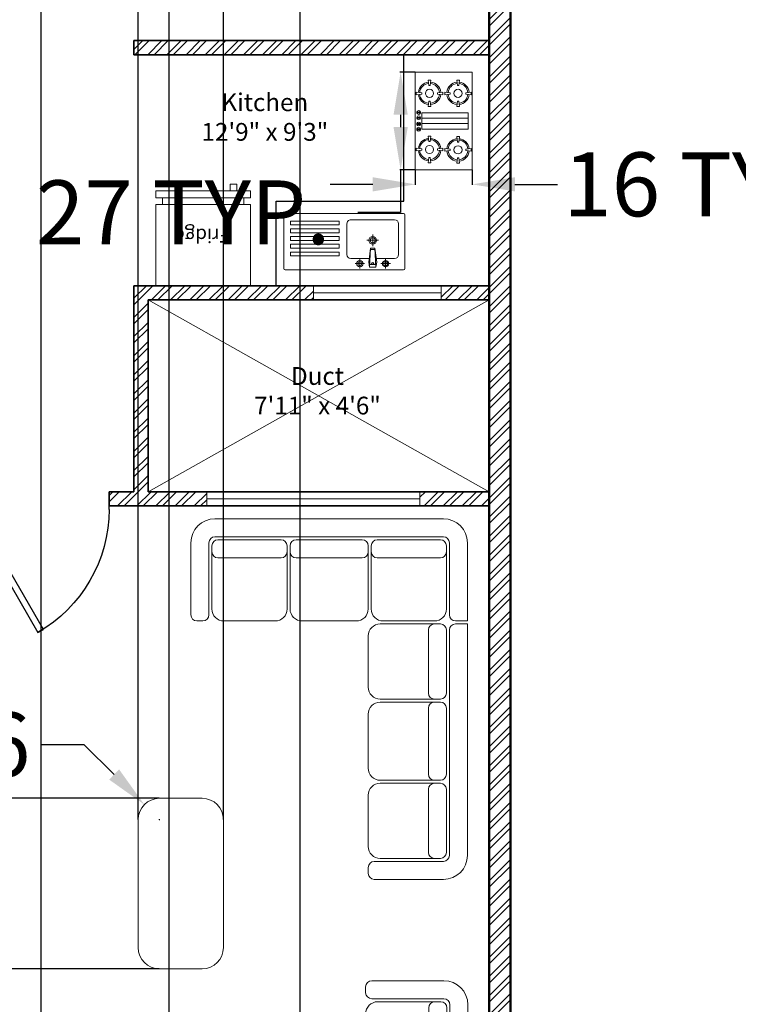
# Model space of a CAD drawing. Units: inches. Extents: x 73 to 1216, y -495 to 328.
# Tile 6 of 9: x 792 to 994, y -232 to 45. Entities that reach past the tile are written whole.
import ezdxf

# ---------------------------------------------------------------- set-up
doc = ezdxf.new("R2010")
doc.units = ezdxf.units.IN
for name, color, linetype, lineweight in [('A-ANNO-DIMS', 2, 'Continuous', 18), ('A-AREA-IDEN', 7, 'Continuous', 18), ('A-DOOR', 3, 'Continuous', 25), ('A-EQPM', 6, 'Continuous', 18), ('A-FLOR-FIXT', 9, 'Continuous', 18), ('A-FLOR-OPEN', 8, 'Continuous', 13), ('A-GLAZ', 3, 'Continuous', 18), ('A-WALL-PATT', 8, 'Continuous', 13), ('Furniture', 2, 'Continuous', 18), ('Inner Walls', 5, 'Continuous', 35), ('Kitchen', 6, 'Continuous', 25), ('Outer Walls', 1, 'Continuous', 50), ('Text-T18', 7, 'Continuous', 18)]:
    doc.layers.add(name, color=color, linetype=linetype, lineweight=lineweight)
doc.styles.get("Standard").update_dxf_attribs({"font": 'arial.ttf'})
doc.dimstyles.get("Standard").update_dxf_attribs({"dimtxt": 18, "dimasz": 12, "dimexe": 0.18, "dimexo": 0.0625, "dimgap": 0.09, "dimtad": 0, "dimtih": 1, "dimtoh": 1, "dimdec": 0, "dimzin": 0, "dimdsep": 46, "dimlunit": 3, "dimtxsty": 'Standard', "dimcen": 0.09, "dimadec": 0, "dimazin": 0, "dimtfac": 1, "dimtdec": 0, "dimtofl": 0, "dimtmove": 0, "dimatfit": 3, "dimfxl": 1, "dimtolj": 1, "dimtzin": 0, "dimarcsym": 0})
pattern_1 = [(45, (-647.324, -1257.0093), (-2.694077, 2.694077), []), (45, (-645.528, -1257.0093), (-2.694077, 2.694077), [])]

# ---------------------------------------------------------------- blocks, each defined once
blk = doc.blocks.new('*U4')
for p, q in [((0, 0), (0, -4)), ((40, 0), (40, -4))]:
    blk.add_line(p, q)
blk.add_lwpolyline([(0, 0), (20, 34.64), (21.52, 33.77), (1.52, -0.88)], close=True)
blk.add_arc((0, 0), 40, 0, 60)
blk = doc.blocks.new('A$C2AFA021D')
for p, q in [((0.8, 2.3), (0.2, 2.3)), ((0.85, 2.2), (0.85, 2.25)), ((0.2, 2.15), (0.8, 2.15)), ((0, 2.1), (0, 0.2)), ((0.15, 0.2), (0.15, 2.1)), ((0.175, 1.55), (0.175, 2.075)), ((0.225, 2.125), (0.275, 2.125)), ((0.75, 2.125), (0.275, 2.125)), ((0.325, 2.075), (0.325, 1.55)), ((0.85, 1.6), (0.85, 2.025)), ((0.275, 1.5), (0.225, 1.5)), ((0.225, 1.475), (0.275, 1.475)), ((0.275, 1.5), (0.75, 1.5)), ((0.75, 1.475), (0.275, 1.475)), ((0.175, 0.875), (0.175, 1.425)), ((0.325, 1.425), (0.325, 0.875)), ((0.85, 0.925), (0.85, 1.375)), ((0.275, 0.825), (0.225, 0.825)), ((0.275, 0.825), (0.75, 0.825)), ((0.975, 0.825), (1.4, 0.825)), ((1.625, 0.825), (2.075, 0.825)), ((2.3, 0.825), (2.725, 0.825)), ((2.9, 0.825), (2.95, 0.825)), ((0.175, 0.225), (0.175, 0.75)), ((0.225, 0.8), (0.275, 0.8)), ((0.75, 0.8), (0.275, 0.8)), ((0.325, 0.75), (0.325, 0.225)), ((2.85, 0.2), (2.85, 0.775)), ((3, 0.775), (3, 0.2)), ((0.85, 0.275), (0.85, 0.7)), ((0.875, 0.275), (0.875, 0.725)), ((1.5, 0.725), (1.5, 0.275)), ((1.525, 0.275), (1.525, 0.725)), ((2.175, 0.725), (2.175, 0.275)), ((2.2, 0.275), (2.2, 0.725)), ((2.825, 0.725), (2.825, 0.275)), ((0.875, 0.275), (0.875, 0.225)), ((1.45, 0.325), (0.925, 0.325)), ((1.5, 0.225), (1.5, 0.275)), ((1.525, 0.275), (1.525, 0.225)), ((2.125, 0.325), (1.575, 0.325)), ((2.175, 0.225), (2.175, 0.275)), ((2.2, 0.275), (2.2, 0.225)), ((2.775, 0.325), (2.25, 0.325)), ((2.825, 0.225), (2.825, 0.275)), ((0.275, 0.175), (0.225, 0.175)), ((0.275, 0.175), (0.75, 0.175)), ((0.925, 0.175), (1.45, 0.175)), ((1.575, 0.175), (2.125, 0.175)), ((2.25, 0.175), (2.775, 0.175)), ((0.8, 0.15), (0.2, 0.15)), ((0.85, 0), (0.85, 0.1)), ((0.875, 0.1), (0.875, 0)), ((0.925, 0.15), (2.8, 0.15)), ((0.2, 0), (0.85, 0)), ((2.8, 0), (0.875, 0))]:
    blk.add_line(p, q)
for centre, radius, start, end in [((0.2, 2.1), 0.2, 90, 180), ((0.8, 2.25), 0.05, 0, 90), ((0.2, 2.1), 0.05, 90, 180), ((0.8, 2.2), 0.05, 270, 0), ((0.225, 2.075), 0.05, 90, 180), ((0.275, 2.075), 0.05, 0, 90), ((0.75, 2.025), 0.1, 0, 90), ((0.75, 1.6), 0.1, 270, 0), ((0.225, 1.55), 0.05, 180, 270), ((0.225, 1.425), 0.05, 90, 180), ((0.275, 1.55), 0.05, 270, 0), ((0.275, 1.425), 0.05, 0, 90), ((0.75, 1.375), 0.1, 360, 90), ((0.75, 0.925), 0.1, 270, 0), ((0.225, 0.875), 0.05, 180, 270), ((0.275, 0.875), 0.05, 270, 0), ((0.975, 0.725), 0.1, 90, 180), ((1.4, 0.725), 0.1, 0, 90), ((1.625, 0.725), 0.1, 90, 180), ((2.075, 0.725), 0.1, 0, 90), ((2.3, 0.725), 0.1, 90, 180), ((2.725, 0.725), 0.1, 0, 90), ((2.9, 0.775), 0.05, 90, 180), ((2.95, 0.775), 0.05, 0, 90), ((0.225, 0.75), 0.05, 90, 180), ((0.275, 0.75), 0.05, 0, 90), ((0.75, 0.7), 0.1, 0, 90), ((0.75, 0.275), 0.1, 270, 0), ((0.925, 0.275), 0.05, 90, 180), ((1.45, 0.275), 0.05, 360, 90), ((1.575, 0.275), 0.05, 90, 180), ((2.125, 0.275), 0.05, 360, 90), ((2.25, 0.275), 0.05, 90, 180), ((2.775, 0.275), 0.05, 360, 90), ((0.2, 0.2), 0.2, 180, 270), ((0.2, 0.2), 0.05, 180, 270), ((0.225, 0.225), 0.05, 180, 270), ((0.275, 0.225), 0.05, 270, 0), ((0.925, 0.225), 0.05, 180, 270), ((1.45, 0.225), 0.05, 270, 0), ((1.575, 0.225), 0.05, 180, 270), ((2.125, 0.225), 0.05, 270, 0), ((2.25, 0.225), 0.05, 180, 270), ((2.775, 0.225), 0.05, 270, 0), ((2.8, 0.2), 0.2, 270, 0), ((2.8, 0.2), 0.05, 270, 0), ((0.8, 0.1), 0.05, 0, 90), ((0.925, 0.1), 0.05, 90, 180)]:
    blk.add_arc(centre, radius, start, end)
blk = doc.blocks.new('A$C57CF26DA')
for p, q in [((0, 0), (0, 420)), ((720, 420), (0, 420)), ((166.9, 413), (146.9, 413)), ((146.9, 413), (151.9, 373)), ((151.9, 373), (161.9, 373)), ((161.9, 373), (166.9, 413)), ((300, 390.9), (300, 49.1)), ((300, 390.9), (420, 390.9)), ((340, 390.9), (340, 49.1)), ((380, 390.9), (380, 49.1)), ((420, 390.9), (420, 49.1)), ((583.6, 413), (563.6, 413)), ((563.6, 413), (568.6, 373)), ((568.6, 373), (578.6, 373)), ((578.6, 373), (583.6, 413)), ((720, 0), (720, 420)), ((98.9, 320), (58.9, 325)), ((58.9, 325), (58.9, 305)), ((58.9, 305), (98.9, 310)), ((98.9, 310), (98.9, 320)), ((254.8, 325), (214.8, 320)), ((214.8, 320), (214.8, 310)), ((214.8, 310), (254.8, 305)), ((254.8, 305), (254.8, 325)), ((515.6, 320), (475.6, 325)), ((475.6, 325), (475.6, 305)), ((475.6, 305), (515.6, 310)), ((515.6, 310), (515.6, 320)), ((671.6, 325), (631.6, 320)), ((631.6, 320), (631.6, 310)), ((631.6, 310), (671.6, 305)), ((671.6, 305), (671.6, 325)), ((151.9, 257), (146.9, 217)), ((161.9, 257), (151.9, 257)), ((166.9, 217), (161.9, 257)), ((568.6, 257), (563.6, 217)), ((578.6, 257), (568.6, 257)), ((583.6, 217), (578.6, 257)), ((146.9, 217), (166.9, 217)), ((166.9, 203), (146.9, 203)), ((146.9, 203), (151.9, 163)), ((151.9, 163), (161.9, 163)), ((161.9, 163), (166.9, 203)), ((581.1, 203), (561.1, 203)), ((561.1, 203), (566.1, 163)), ((563.6, 217), (583.6, 217)), ((566.1, 163), (576.1, 163)), ((576.1, 163), (581.1, 203)), ((98.9, 110), (58.9, 115)), ((58.9, 115), (58.9, 95)), ((58.9, 95), (98.9, 100)), ((98.9, 100), (98.9, 110)), ((254.8, 115), (214.8, 110)), ((214.8, 110), (214.8, 100)), ((214.8, 100), (254.8, 95)), ((254.8, 95), (254.8, 115)), ((513.1, 110), (473.1, 115)), ((473.1, 115), (473.1, 95)), ((473.1, 95), (513.1, 100)), ((513.1, 100), (513.1, 110)), ((669, 115), (629, 110)), ((629, 110), (629, 100)), ((629, 100), (669, 95)), ((669, 95), (669, 115)), ((151.9, 47), (146.9, 7)), ((146.9, 7), (166.9, 7)), ((161.9, 47), (151.9, 47)), ((166.9, 7), (161.9, 47)), ((301.5, 38.7), (294.7, 38.7)), ((294.7, 38.7), (294.7, 11.3)), ((294.7, 11.3), (301.5, 11.3)), ((420, 49.1), (300, 49.1)), ((301.5, 11.3), (301.5, 38.7)), ((340.5, 38.7), (333.7, 38.7)), ((333.7, 38.7), (333.7, 11.3)), ((333.7, 11.3), (340.5, 11.3)), ((340.5, 11.3), (340.5, 38.7)), ((379.7, 11.3), (379.7, 38.7)), ((379.7, 38.7), (386.5, 38.7)), ((386.5, 11.3), (379.7, 11.3)), ((386.5, 38.7), (386.5, 11.3)), ((418.7, 11.3), (418.7, 38.7)), ((418.7, 38.7), (425.5, 38.7)), ((425.5, 11.3), (418.7, 11.3)), ((425.5, 38.7), (425.5, 11.3)), ((566.1, 47), (561.1, 7)), ((561.1, 7), (581.1, 7)), ((576.1, 47), (566.1, 47)), ((581.1, 7), (576.1, 47)), ((720, 0), (0, 0))]:
    blk.add_line(p, q)
for centre in [(156.9, 315), (573.6, 315), (156.9, 105), (571.1, 105)]:
    blk.add_circle(centre, 30)
for centre, radius, start, end in [((156.9, 315), 83, 95.58493, 174.41507), ((156.9, 315), 73, 95.37384, 174.62616), ((156.9, 315), 73, 5.37384, 84.62616), ((156.9, 315), 83, 5.58493, 84.41507), ((573.6, 315), 83, 95.58493, 174.41507), ((573.6, 315), 73, 95.37384, 174.62616), ((573.6, 315), 73, 5.37384, 84.62616), ((573.6, 315), 83, 5.58493, 84.41507), ((156.9, 315), 83, 185.58493, 264.41507), ((156.9, 315), 73, 185.37384, 264.62616), ((156.9, 315), 73, 275.37384, 354.62616), ((156.9, 315), 83, 275.58493, 354.41507), ((573.6, 315), 83, 185.58493, 264.41507), ((573.6, 315), 73, 185.37384, 264.62616), ((573.6, 315), 73, 275.37384, 354.62616), ((573.6, 315), 83, 275.58493, 354.41507), ((156.9, 105), 83, 95.58493, 174.41507), ((156.9, 105), 73, 95.37384, 174.62616), ((156.9, 105), 73, 5.37384, 84.62616), ((156.9, 105), 83, 5.58493, 84.41507), ((571.1, 105), 83, 95.58493, 174.41507), ((571.1, 105), 73, 95.37384, 174.62616), ((571.1, 105), 73, 5.37384, 84.62616), ((571.1, 105), 83, 5.58493, 84.41507), ((156.9, 105), 83, 185.58493, 264.41507), ((156.9, 105), 73, 185.37384, 264.62616), ((156.9, 105), 73, 275.37384, 354.62616), ((156.9, 105), 83, 275.58493, 354.41507), ((571.1, 105), 83, 185.58493, 264.41507), ((571.1, 105), 73, 185.37384, 264.62616), ((571.1, 105), 73, 275.37384, 354.62616), ((571.1, 105), 83, 275.58493, 354.41507), ((298.1, 25), 13.7, 104.47751, 255.52249), ((298.1, 25), 13.7, 284.47751, 75.52249), ((337.1, 25), 13.7, 104.47751, 255.52249), ((337.1, 25), 13.7, 284.47751, 75.52249), ((383.1, 25), 13.7, 104.47751, 255.52249), ((383.1, 25), 13.7, 284.47751, 75.52249), ((422.1, 25), 13.7, 104.47751, 255.52249), ((422.1, 25), 13.7, 284.47751, 75.52249)]:
    blk.add_arc(centre, radius, start, end)
blk = doc.blocks.new('A$C7C492201')
for p, q in [((0, 10), (0, 426.6)), ((10, 436.6), (927.3, 436.6)), ((111.9, 388.7), (185, 388.7)), ((148.5, 425.2), (148.5, 352.2)), ((223.5, 415), (217, 376.2)), ((223.5, 415), (231.8, 268.5)), ((223.5, 415), (248.5, 415)), ((224.6, 395.4), (248.5, 395.4)), ((273.5, 415), (248.5, 415)), ((272.3, 395.4), (248.5, 395.4)), ((273.5, 415), (265.2, 268.5)), ((273.5, 415), (279.9, 376.2)), ((311.9, 388.7), (385, 388.7)), ((348.5, 425.2), (348.5, 352.2)), ((937.3, 10), (937.3, 426.6)), ((48.5, 318.8), (48.5, 78.8)), ((220.8, 348.8), (78.5, 348.8)), ((217, 376.2), (231.8, 268.5)), ((279.9, 376.2), (265.2, 268.5)), ((418.5, 348.8), (276.2, 348.8)), ((448.5, 318.8), (448.5, 78.8)), ((509.1, 328.4), (509.1, 298.4)), ((509.1, 328.4), (885, 328.4)), ((885, 328.4), (885, 298.4)), ((231.3, 278.6), (248.5, 278.6)), ((231.8, 268.5), (248.5, 268.5)), ((265.6, 278.6), (248.5, 278.6)), ((265.2, 268.5), (248.5, 268.5)), ((248.5, 252.8), (248.5, 162.6)), ((509.1, 298.4), (885, 298.4)), ((509.1, 268.4), (509.1, 238.4)), ((509.1, 268.4), (885, 268.4)), ((509.1, 238.4), (885, 238.4)), ((885, 268.4), (885, 238.4)), ((203.4, 207.7), (293.5, 207.7)), ((509.1, 208.4), (885, 208.4)), ((509.1, 208.4), (509.1, 178.4)), ((509.1, 178.4), (885, 178.4)), ((885, 208.4), (885, 178.4)), ((509.1, 148.4), (509.1, 118.4)), ((509.1, 148.4), (885, 148.4)), ((509.1, 118.4), (885, 118.4)), ((509.1, 88.4), (509.1, 58.4)), ((509.1, 88.4), (885, 88.4)), ((885, 148.4), (885, 118.4)), ((885, 88.4), (885, 58.4)), ((927.3, 0), (10, 0)), ((418.5, 48.8), (78.5, 48.8)), ((509.1, 58.4), (885, 58.4))]:
    blk.add_line(p, q)
for centre, radius in [((148.5, 388.7), 25), ((148.5, 388.7), 15), ((348.5, 388.7), 25), ((348.5, 388.7), 15), ((248.5, 207.7), 30), ((248.5, 207.7), 20)]:
    blk.add_circle(centre, radius)
for centre, radius, start, end in [((10, 426.6), 10, 90, 180), ((247.3, 388), 7.19, 80.52523, 279.47477), ((249.6, 388), 7.19, 260.52523, 99.47477), ((927.3, 426.6), 10, 0, 90), ((78.5, 318.8), 30, 90, 180), ((418.5, 318.8), 30, 0, 90), ((78.5, 78.8), 30, 180, 270), ((418.5, 78.8), 30, 270, 0), ((10, 10), 10, 180, 270), ((927.3, 10), 10, 270, 0)]:
    blk.add_arc(centre, radius, start, end)
blk = doc.blocks.new('REFRI-00')
for points in [[(-0.35, 0.35), (-0.35, -0.25), (0.35, -0.25), (0.35, 0.35), (-0.35, 0.35)], [(-0.3, -0.3), (-0.3, -0.25)], [(0.3, -0.3), (0.3, -0.25)], [(-0.35, -0.3), (-0.35, -0.35), (0.35, -0.35), (0.35, -0.3), (-0.35, -0.3)], [(-0.25, -0.35), (-0.25, -0.4), (-0.2, -0.4), (-0.2, -0.35)]]:
    blk.add_lwpolyline(points)
blk = doc.blocks.new('*D26')
at = {"layer": 'A-ANNO-DIMS', "color": 0, "lineweight": -2, "transparency": 16777216}
for p, q in [((690.69, 91.4), (690.69, 79.21)), ((771.16, 91.4), (771.16, 79.21)), ((702.69, 79.39), (759.16, 79.39)), ((771.16, 79.39), (783.16, 79.39))]:
    blk.add_line(p, q, dxfattribs=at)
at = {"layer": 'A-ANNO-DIMS', "color": 0, "transparency": 16777216}
for points in [[(702.69, 81.39), (702.69, 77.39), (690.69, 79.39)], [(759.16, 81.39), (759.16, 77.39), (771.16, 79.39)]]:
    blk.add_solid(points, dxfattribs=at)
at = {"layer": 'Defpoints', "color": 0, "transparency": 16777216}
for p in [(690.69, 91.46), (771.16, 91.46), (771.16, 79.39)]:
    blk.add_point(p, dxfattribs=at)
at = {"layer": 'A-ANNO-DIMS', "color": 0, "transparency": 16777216, "insert": (890.24, 79.39), "char_height": 18, "attachment_point": 5}
blk.add_mtext('\\A1;KING BED 80 TYP.', dxfattribs=at)
blk = doc.blocks.new('*D38')
at = {"layer": 'A-ANNO-DIMS', "color": 0, "lineweight": -2, "transparency": 16777216}
for p, q in [((835.16, 83.11), (835.16, 69.65)), ((924.16, 83.11), (924.16, 69.65)), ((847.16, 69.83), (912.16, 69.83)), ((924.16, 69.83), (936.16, 69.83))]:
    blk.add_line(p, q, dxfattribs=at)
at = {"layer": 'A-ANNO-DIMS', "color": 0, "transparency": 16777216}
for points in [[(847.16, 71.83), (847.16, 67.83), (835.16, 69.83)], [(912.16, 71.83), (912.16, 67.83), (924.16, 69.83)]]:
    blk.add_solid(points, dxfattribs=at)
at = {"layer": 'Defpoints', "color": 0, "transparency": 16777216}
for p in [(835.16, 83.18), (924.16, 83.18), (924.16, 69.83)]:
    blk.add_point(p, dxfattribs=at)
at = {"layer": 'A-ANNO-DIMS', "color": 0, "transparency": 16777216, "insert": (1057.97, 69.83), "char_height": 18, "attachment_point": 5}
blk.add_mtext('\\A1;WARDROBE 89 TYP.', dxfattribs=at)
blk = doc.blocks.new('*D42')
at = {"layer": 'A-ANNO-DIMS', "color": 0, "lineweight": -2, "transparency": 16777216}
for p, q in [((903.29, 30.3), (899.05, 30.3)), ((899.23, 18.3), (899.23, 14.82)), ((903.29, 2.82), (899.05, 2.82)), ((899.23, 2.82), (899.23, -9.18)), ((899.23, -9.18), (887.23, -9.18))]:
    blk.add_line(p, q, dxfattribs=at)
at = {"layer": 'A-ANNO-DIMS', "color": 0, "transparency": 16777216}
for points in [[(897.23, 18.3), (901.23, 18.3), (899.23, 30.3)], [(897.23, 14.82), (901.23, 14.82), (899.23, 2.82)]]:
    blk.add_solid(points, dxfattribs=at)
at = {"layer": 'Defpoints', "color": 0, "transparency": 16777216}
for p in [(903.36, 30.3), (899.23, 2.82), (903.36, 2.82)]:
    blk.add_point(p, dxfattribs=at)
at = {"layer": 'A-ANNO-DIMS', "color": 0, "transparency": 16777216, "insert": (777.07, -9.18), "char_height": 18, "attachment_point": 5}
blk.add_mtext('\\A1;COOKTOP 27 TYP.', dxfattribs=at)
blk = doc.blocks.new('*D43')
at = {"layer": 'A-ANNO-DIMS', "color": 0, "lineweight": -2, "transparency": 16777216}
for p, q in [((903.36, 2.76), (903.36, -1.48)), ((919.39, 2.76), (919.39, -1.48)), ((891.36, -1.3), (879.36, -1.3)), ((931.39, -1.3), (943.39, -1.3))]:
    blk.add_line(p, q, dxfattribs=at)
at = {"layer": 'A-ANNO-DIMS', "color": 0, "transparency": 16777216}
for points in [[(891.36, 0.7), (891.36, -3.3), (903.36, -1.3)], [(931.39, 0.7), (931.39, -3.3), (919.39, -1.3)]]:
    blk.add_solid(points, dxfattribs=at)
at = {"layer": 'Defpoints', "color": 0, "transparency": 16777216}
for p in [(903.36, 2.82), (919.39, 2.82), (919.39, -1.3)]:
    blk.add_point(p, dxfattribs=at)
at = {"layer": 'A-ANNO-DIMS', "color": 0, "transparency": 16777216, "insert": (986.44, -1.3), "char_height": 18, "attachment_point": 5}
blk.add_mtext('\\A1;16 TYP.', dxfattribs=at)
blk = doc.blocks.new('*D67')
at = {"layer": 'A-ANNO-DIMS', "color": 0, "lineweight": -2, "transparency": 16777216}
for p, q in [((798.02113, 227.113801), (798.02113, -465.403699)), ((834.02113, 227.113801), (834.02113, -465.403699)), ((786.02113, -465.223699), (774.02113, -465.223699)), ((846.02113, -465.223699), (858.02113, -465.223699))]:
    blk.add_line(p, q, dxfattribs=at)
at = {"layer": 'A-ANNO-DIMS', "color": 0, "transparency": 16777216}
for points in [[(786.02113, -463.223699), (786.02113, -467.223699), (798.02113, -465.223699)], [(846.02113, -463.223699), (846.02113, -467.223699), (834.02113, -465.223699)]]:
    blk.add_solid(points, dxfattribs=at)
at = {"layer": 'Defpoints', "color": 0, "transparency": 16777216}
for p in [(798.02113, 227.176301), (834.02113, 227.176301), (834.02113, -465.223699)]:
    blk.add_point(p, dxfattribs=at)
at = {"layer": 'A-ANNO-DIMS', "color": 0, "transparency": 16777216, "insert": (816.02113, -465.223699), "char_height": 18, "attachment_point": 5}
blk.add_mtext('\\A1;36', dxfattribs=at)
blk = doc.blocks.new('*D68')
at = {"layer": 'A-ANNO-DIMS', "color": 0, "lineweight": -2, "transparency": 16777216}
for p, q in [((834.02, 227.11), (834.02, -465.4)), ((870.82, 227.11), (870.82, -465.4)), ((846.02, -465.22), (858.82, -465.22)), ((870.82, -465.22), (882.82, -465.22))]:
    blk.add_line(p, q, dxfattribs=at)
at = {"layer": 'A-ANNO-DIMS', "color": 0, "transparency": 16777216}
for points in [[(846.02, -463.22), (846.02, -467.22), (834.02, -465.22)], [(858.82, -463.22), (858.82, -467.22), (870.82, -465.22)]]:
    blk.add_solid(points, dxfattribs=at)
at = {"layer": 'Defpoints', "color": 0, "transparency": 16777216}
for p in [(834.02, 227.18), (870.82, 227.18), (870.82, -465.22)]:
    blk.add_point(p, dxfattribs=at)
at = {"layer": 'A-ANNO-DIMS', "color": 0, "transparency": 16777216, "insert": (906.3, -465.22), "char_height": 18, "attachment_point": 5}
blk.add_mtext('\\A1;36.8', dxfattribs=at)
blk = doc.blocks.new('*D77')
at = {"layer": 'A-ANNO-DIMS', "color": 0, "lineweight": -2, "transparency": 16777216}
for p, q in [((813.36, 316.58), (801.36, 316.58)), ((825.36, -180.08), (825.36, 316.76)), ((849.36, -180.08), (849.36, 316.76)), ((861.36, 316.58), (873.36, 316.58))]:
    blk.add_line(p, q, dxfattribs=at)
at = {"layer": 'A-ANNO-DIMS', "color": 0, "transparency": 16777216}
for points in [[(813.36, 318.58), (813.36, 314.58), (825.36, 316.58)], [(861.36, 318.58), (861.36, 314.58), (849.36, 316.58)]]:
    blk.add_solid(points, dxfattribs=at)
at = {"layer": 'Defpoints', "color": 0, "transparency": 16777216}
for p in [(849.36, 316.58), (825.36, -180.14), (849.36, -180.14)]:
    blk.add_point(p, dxfattribs=at)
at = {"layer": 'A-ANNO-DIMS', "color": 0, "transparency": 16777216, "insert": (886.46, 316.58), "char_height": 18, "attachment_point": 5}
blk.add_mtext('\\A1;24', dxfattribs=at)
blk = doc.blocks.new('*D78')
at = {"layer": 'A-ANNO-DIMS', "color": 0, "lineweight": -2, "transparency": 16777216}
for p, q in [((831.3, -174.14), (542.58, -174.14)), ((542.76, -186.14), (542.76, -188.86)), ((542.76, -210.14), (542.76, -207.42)), ((831.3, -222.14), (542.58, -222.14))]:
    blk.add_line(p, q, dxfattribs=at)
at = {"layer": 'A-ANNO-DIMS', "color": 0, "transparency": 16777216}
for points in [[(540.76, -186.14), (544.76, -186.14), (542.76, -174.14)], [(540.76, -210.14), (544.76, -210.14), (542.76, -222.14)]]:
    blk.add_solid(points, dxfattribs=at)
at = {"layer": 'Defpoints', "color": 0, "transparency": 16777216}
for p in [(542.76, -174.14), (831.36, -174.14), (831.36, -222.14)]:
    blk.add_point(p, dxfattribs=at)
at = {"layer": 'A-ANNO-DIMS', "color": 0, "transparency": 16777216, "insert": (542.76, -198.14), "char_height": 18, "attachment_point": 5}
blk.add_mtext('\\A1;48', dxfattribs=at)
blk = doc.blocks.new('*D79')
at = {"layer": 'A-ANNO-DIMS', "color": 0, "lineweight": -2, "transparency": 16777216}
for p, q in [((798.1, -158.97), (810.1, -158.97)), ((810.1, -158.97), (818.61, -167.44)), ((831.27, -180.14), (831.45, -180.14)), ((831.36, -180.23), (831.36, -180.05))]:
    blk.add_line(p, q, dxfattribs=at)
at = {"layer": 'A-ANNO-DIMS', "color": 0, "transparency": 16777216}
blk.add_solid([(820.02, -166.02), (817.19, -168.86), (827.11, -175.91)], dxfattribs=at)
at = {"layer": 'Defpoints', "color": 0, "transparency": 16777216}
for p in [(827.11, -175.91), (831.36, -180.14)]:
    blk.add_point(p, dxfattribs=at)
at = {"layer": 'A-ANNO-DIMS', "color": 0, "transparency": 16777216, "insert": (763.81, -158.97), "char_height": 18, "attachment_point": 5}
blk.add_mtext('\\A1;4X R6', dxfattribs=at)

msp = doc.modelspace()

# ---------------------------------------------------------------- hatches: boundary and pattern name
at = {"layer": 'A-WALL-PATT'}
h = msp.add_hatch(dxfattribs=at)
h.set_pattern_fill('ANSI32', color=256, scale=0.4)
h.set_pattern_definition(pattern_1)
h.paths.add_polyline_path([(586.1647, 273.1763), (924.1647, 273.1763), (924.1647, -421.8237), (753.1647, -421.8237), (753.1647, -427.8237), (930.1647, -427.8237), (930.1647, 279.1763), (580.1647, 279.1763), (580.1647, -427.8237), (633.1647, -427.8237), (633.1647, -421.8237), (586.1647, -421.8237)])
h = msp.add_hatch(dxfattribs=at)
h.set_pattern_fill('ANSI32', color=256, scale=0.4)
h.set_pattern_definition(pattern_1)
h.paths.add_polyline_path([(685.1647, 201.1763), (679.1647, 201.1763), (679.1647, 206.1763), (675.1647, 206.1763), (675.1647, 201.1763), (586.1647, 201.1763), (586.1647, 197.1763), (685.1647, 197.1763)])
h.paths.add_polyline_path([(679.1647, 273.1763), (675.1647, 273.1763), (675.1647, 236.1763), (679.1647, 236.1763)])
h.paths.add_polyline_path([(775.1647, 201.1763), (772.1647, 201.1763), (772.1647, 273.1763), (768.1647, 273.1763), (768.1647, 249.1763), (768.1647, 201.1763), (721.1647, 201.1763), (721.1647, 197.1763), (771.1647, 197.1763), (771.1647, 58.1763), (775.1647, 58.1763)])
h.paths.add_polyline_path([(798.0211, 233.1763), (772.1647, 233.1763), (772.1647, 227.1763), (798.0211, 227.1763)])
h.paths.add_polyline_path([(870.8232, 233.1763), (834.0211, 233.1763), (834.0211, 227.1763), (870.8232, 227.1763)])
h.paths.add_polyline_path([(924.1647, 233.1763), (906.8232, 233.1763), (906.8232, 227.1763), (924.1647, 227.1763)])
h.paths.add_polyline_path([(924.1647, 83.1763), (775.1647, 83.1763), (775.1647, 79.1763), (924.1647, 79.1763)])
h.paths.add_polyline_path([(775.1647, 22.1763), (771.1647, 22.1763), (771.1647, 16.1763), (628.1647, 16.1763), (628.1647, 12.1763), (775.1647, 12.1763)])
h.paths.add_polyline_path([(692.1647, 12.1763), (688.1647, 12.1763), (688.1647, -52.8237), (692.1647, -52.8237)])
h.paths.add_polyline_path([(924.1647, 39.1763), (824.1647, 39.1763), (824.1647, 35.1763), (924.1647, 35.1763)])
h.paths.add_polyline_path([(874.6647, -29.8237), (864.1647, -29.8237), (824.1647, -29.8237), (824.1647, -87.8237), (817.1647, -87.8237), (817.1647, -91.8237), (844.6647, -91.8237), (844.6647, -87.8237), (828.1647, -87.8237), (828.1647, -33.8237), (874.6647, -33.8237)])
h.paths.add_polyline_path([(924.1647, -29.8237), (910.6647, -29.8237), (910.6647, -33.8237), (924.1647, -33.8237)])
h.paths.add_polyline_path([(924.1647, -87.8237), (904.6647, -87.8237), (904.6647, -91.8237), (924.1647, -91.8237)])
h.paths.add_polyline_path([(777.1647, -88.8237), (761.1647, -88.8237), (761.1647, -92.8237), (767.1647, -92.8237), (767.1647, -224.8237), (771.1647, -224.8237), (771.1647, -92.8237), (777.1647, -92.8237)])
h.paths.add_polyline_path([(725.1647, -88.8237), (628.1647, -88.8237), (628.1647, -92.8237), (725.1647, -92.8237)])
h.paths.add_polyline_path([(692.1647, -82.8237), (688.1647, -82.8237), (688.1647, -88.8237), (692.1647, -88.8237)])
h.paths.add_polyline_path([(767.1647, -313.8237), (924.1647, -313.8237), (924.1647, -307.8237), (763.1647, -307.8237), (763.1647, -421.8237), (767.1647, -421.8237)])

# ---------------------------------------------------------------- linework, layer by layer
at = {"layer": 'A-FLOR-OPEN'}
for p, q in [((828.1647, -87.8237), (924.1647, -33.8237)), ((828.1647, -33.8237), (924.1647, -87.8237))]:
    msp.add_line(p, q, dxfattribs=at)
at = {"layer": 'A-GLAZ'}
for p, q in [((874.6647, -33.8237), (874.6647, -29.8237)), ((910.6647, -33.8237), (910.6647, -29.8237)), ((910.6647, -31.8237), (874.6647, -31.8237)), ((844.6647, -91.8237), (844.6647, -87.8237)), ((904.6647, -91.8237), (904.6647, -87.8237)), ((904.6647, -89.8237), (844.6647, -89.8237))]:
    msp.add_line(p, q, dxfattribs=at)
at = {"layer": 'Furniture'}
msp.add_lwpolyline([(831.3578, -174.1414), (843.3578, -174.1414, -0.41421356), (849.3578, -180.1414), (849.3578, -216.1414, -0.41421356), (843.3578, -222.1414), (831.3578, -222.1414, -0.41421356), (825.3578, -216.1414), (825.3578, -180.1414, -0.41421356)], format="xyb", close=True, dxfattribs=at)
at = {"layer": 'Inner Walls'}
for p, q in [((824.1647, 39.1763), (924.1647, 39.1763)), ((824.1647, 39.1763), (824.1647, 35.1763)), ((824.1647, 35.1763), (924.1647, 35.1763)), ((924.1647, -29.8237), (824.1647, -29.8237)), ((824.1647, -87.8237), (824.1647, -29.8237)), ((924.1647, -33.8237), (828.1647, -33.8237)), ((828.1647, -87.8237), (828.1647, -33.8237)), ((824.1647, -87.8237), (817.1647, -87.8237)), ((817.1647, -87.8237), (817.1647, -91.8237)), ((924.1647, -87.8237), (828.1647, -87.8237)), ((924.1647, -91.8237), (817.1647, -91.8237))]:
    msp.add_line(p, q, dxfattribs=at)
at = {"layer": 'Kitchen'}
msp.add_lwpolyline([(864.1647, -6.0549), (900.1647, -6.0549), (900.1647, 35.1763), (924.1647, 35.1763), (924.1647, -29.8237), (864.1647, -29.8237)], close=True, dxfattribs=at)
at = {"layer": 'Outer Walls'}
for p, q in [((930.1647, -427.8237), (930.1647, 279.1763)), ((924.1647, -421.8237), (924.1647, 273.1763))]:
    msp.add_line(p, q, dxfattribs=at)

# ---------------------------------------------------------------- block references
at = {"layer": 'A-DOOR', "xscale": -1, "rotation": 180}
msp.add_blockref('*U4', (777.1647, -92.8237), dxfattribs=at)
at = {"layer": 'A-EQPM'}
for name, p, xscale, yscale, zscale, rotation in [('A$C57CF26DA', (903.3556, 30.303), 0.0381707681172169, 0.0381707681172169, 0.0381707681172169, 270), ('REFRI-00', (843.6515, -16.491), 38.0932829071003, 38.0932829071003, 38.0932829071003, 180)]:
    msp.add_blockref(name, p, dxfattribs=dict(at, xscale=xscale, yscale=yscale, zscale=zscale, rotation=rotation))
at = {"layer": 'A-FLOR-FIXT', "xscale": 0.0362851414289068, "yscale": 0.0362851414289068, "zscale": 0.0362851414289068, "rotation": 180}
msp.add_blockref('A$C7C492201', (900.3933, -9.5164), dxfattribs=at)
at = {"layer": 'Furniture', "xscale": -33.84012530478223, "yscale": 33.84012530478223, "zscale": 33.84012530478223, "rotation": 90}
msp.add_blockref('A$C2AFA021D', (918.0312, -95.4493), dxfattribs=at)
at = {"layer": 'Furniture', "xscale": -33.84012530478223, "yscale": 33.84012530478223, "zscale": 33.84012530478223}
msp.add_blockref('A$C2AFA021D', (918.1526, -303.3147), dxfattribs=at)

# ---------------------------------------------------------------- texts
at = {"layer": 'A-AREA-IDEN', "char_height": 5, "attachment_point": 3}
for s, width, insert in [('\\pxqc;{\\fTimes New Roman|b0|i0|c0|p18;Kitchen\\P12\'9" x 9\'3"}', 49.101878, (885.5659, 24.3095)), ('\\pxqc;{\\fTimes New Roman|b0|i0|c0|p18;Duct\\P7\'11" x 4\'6"}', 37.203385, (894.4307, -52.7501))]:
    msp.add_mtext_dynamic_manual_height_columns(s, width=width, gutter_width=12.5, heights=[0], dxfattribs=dict(at, insert=insert))
at = {"layer": 'Text-T18', "insert": (852.3262, -17.6738), "char_height": 3.877971, "attachment_point": 1, "rotation": 180}
msp.add_mtext_dynamic_manual_height_columns('\\pxqc;{\\fTimes New Roman|b0|i0|c0|p18;Fridge}', width=17.951771, gutter_width=4.8475, heights=[0], dxfattribs=at)

# ---------------------------------------------------------------- dimensions: what is measured, and where the dimension line sits
at = {"layer": 'A-ANNO-DIMS'}
for base, p1, p2, override, picture, middle in [((849.3578, 316.5763), (825.3578, -180.1414), (849.3578, -180.1414), {"dimdec": 0, "dimlfac": 1, "dimrnd": 0, "dimzin": 0, "dimdsep": 46, "dimlunit": 2}, '*D77', (886.4567, 316.5763)), ((834.0211, -465.2237), (798.0211, 227.1763), (834.0211, 227.1763), {"dimdec": 0, "dimlfac": 1, "dimrnd": 0, "dimzin": 0, "dimdsep": 46, "dimlunit": 2}, '*D67', (816.0211, -465.2237)), ((870.8232, -465.2237), (834.0211, 227.1763), (870.8232, 227.1763), {"dimdec": 1, "dimlfac": 1, "dimrnd": 0, "dimzin": 0, "dimdsep": 46, "dimlunit": 2}, '*D68', (906.3033, -465.2237))]:
    dim = msp.add_linear_dim(base=base, p1=p1, p2=p2, dimstyle='Standard', override=override, dxfattribs=at)
    dim.commit()
    dim.dimension.update_dxf_attribs({"geometry": picture, "text_midpoint": middle})
for base, p1, p2, text, picture, middle in [((771.1647, 79.3929), (690.6924, 91.4638), (771.1647, 91.4638), 'KING BED <> TYP.', '*D26', (890.2417, 79.3929)), ((924.1647, 69.8263), (835.1647, 83.1763), (924.1647, 83.1763), 'WARDROBE <> TYP.', '*D38', (1057.9696, 69.8263)), ((919.3873, -1.3024), (903.3556, 2.82), (919.3873, 2.82), '<> TYP.', '*D43', (986.4391, -1.3024))]:
    dim = msp.add_linear_dim(base=base, p1=p1, p2=p2, text=text, dimstyle='Standard', override={"dimdec": 0, "dimlfac": 1, "dimrnd": 0, "dimzin": 0, "dimdsep": 46, "dimlunit": 2}, dxfattribs=at)
    dim.commit()
    dim.dimension.update_dxf_attribs({"geometry": picture, "text_midpoint": middle})
dim = msp.add_linear_dim(base=(899.2332, 2.82), p1=(903.3556, 30.303), p2=(903.3556, 2.82), angle=270, text='COOKTOP <> TYP.', dimstyle='Standard', override={"dimdec": 0, "dimlfac": 1, "dimrnd": 0, "dimzin": 0, "dimdsep": 46, "dimlunit": 2}, dxfattribs=at)
dim.commit()
dim.dimension.update_dxf_attribs({"geometry": '*D42', "text_midpoint": (777.0743, -9.18)})
dim = msp.add_radius_dim(center=(831.3578, -180.1414), mpoint=(827.107, -175.9069), text='4X <>', dimstyle='Standard', override={"dimdec": 0, "dimlfac": 1, "dimrnd": 0, "dimzin": 0, "dimdsep": 46, "dimlunit": 2}, dxfattribs=at)
dim.commit()
dim.dimension.update_dxf_attribs({"geometry": '*D79', "text_midpoint": (763.8062, -158.9692)})
dim = msp.add_linear_dim(base=(542.7647, -174.1414), p1=(831.3578, -222.1414), p2=(831.3578, -174.1414), angle=90, dimstyle='Standard', override={"dimdec": 0, "dimlfac": 1, "dimrnd": 0, "dimzin": 0, "dimdsep": 46, "dimlunit": 2}, dxfattribs=at)
dim.commit()
dim.dimension.update_dxf_attribs({"geometry": '*D78', "text_midpoint": (542.7647, -198.1414)})

doc.saveas('drawing.dxf')
